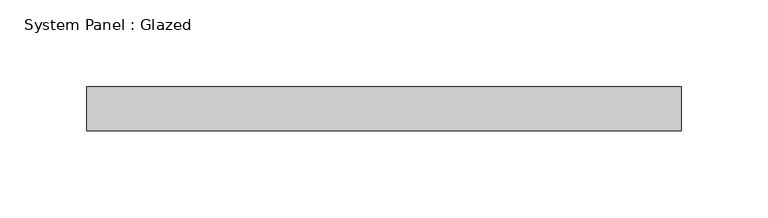
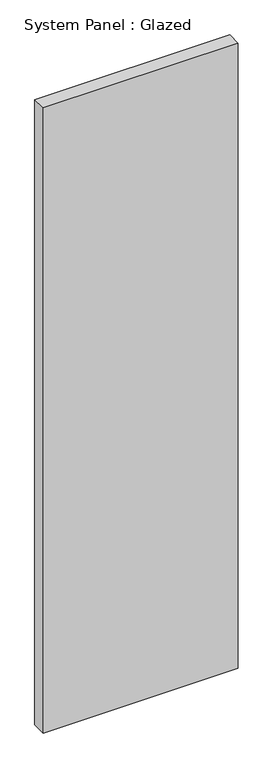
"""IFC4 building model written with IfcOpenShell, lengths in millimetres: plate geometry, System Panel : Glazed."""

from ifc_helpers import new_model, si_unit, origin, origin_with_axes, place, context, project, spatial, polyline, outline, extrude, source, transform, mapped, element, save


def system_panel_glazed_44434818(model_context):
    return source(origin(), model_context, "Body", "SweptSolid", [
        extrude(outline(polyline([(171.45, 19.05), (-171.45, 19.05), (-171.45, 44.45), (171.45, 44.45), (171.45, 19.05)])), origin_with_axes(), (0.0, 0.0, 1.0), 1161.0294817),
    ])


if __name__ == "__main__":
    model = new_model("IFC4")
    model_context = context("Model", 3, world=origin())
    ifc_project = project(units=[si_unit("LENGTHUNIT", "METRE", prefix="MILLI")], contexts=[model_context])
    site = spatial("IfcSite", under=ifc_project)
    building = spatial("IfcBuilding", under=site)
    placement = place(None, origin())
    system_panel_glazed_shape = system_panel_glazed_44434818(model_context)
    element("IfcPlate", 1, ObjectType="System Panel : Glazed", at=placement, inside=building, context=model_context, shape_type="MappedRepresentation", body=[
        mapped(system_panel_glazed_shape, transform((0.0, 0.0, 0.0), x_axis=(1.0, 0.0, 0.0), y_axis=(0.0, 1.0, 0.0), z_axis=(0.0, 0.0, 1.0))),
    ])
    save(model, "model.ifc")

# Revit data of these elements
# Type "System Panel : Glazed"
#   Construction Type Id = "GSP4R"
#   Analytic Construction = "1/8 in Pilkington single glazing"
#   Visual Light Transmittance = 0.9
#   Solar Heat Gain Coefficient = 0.86
#   Heat Transfer Coefficient (U) = 1.18115 BTU/(h·ft²·°F)
#   Define Thermal Properties by = 1
# Element 1 (IfcPlate, "System Panel : Glazed")
#   Materials on its faces: "Glass"
# Materials
#   "Glass": class "Glass", colour RGB 0 128 192, transparency 0.75, Description = "Soda Lime Glass", Cost = 0
